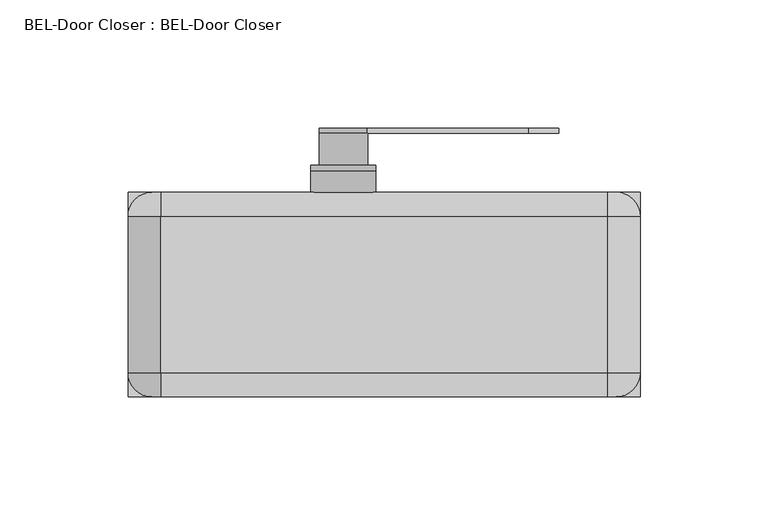
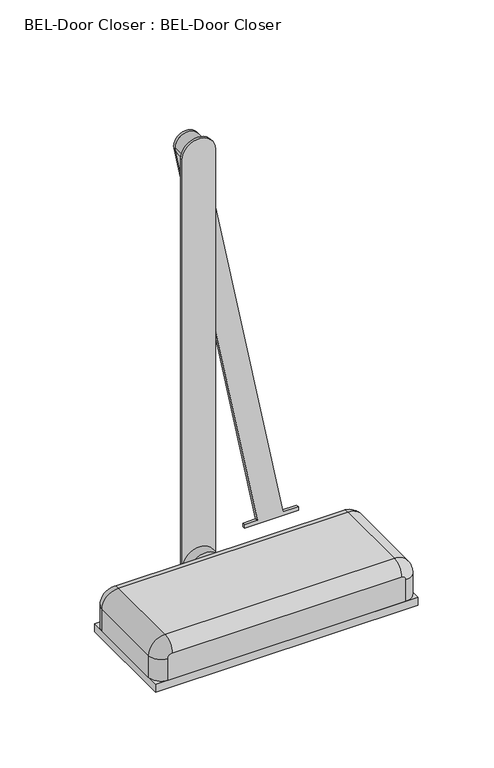
"""IFC4 building model written with IfcOpenShell, lengths in millimetres: proxy geometry, BEL-Door Closer : BEL-Door Closer."""

from ifc_helpers import new_model, si_unit, point, frame, frame_2d, origin, origin_with_axes, place, context, project, spatial, polyline, circle_curve, ellipse_curve, trimmed, segment, composite_curve, outline, extrude, source, transform, mapped, element, save
from ifc_brep_helpers import plane_surface, cylinder_surface, revolved_surface, advanced_brep


def bel_door_closer_bel_door_closer_a3520c2f(model_context):
    return source(origin(), model_context, "Body", "SolidModel", [
        extrude(outline(composite_curve([segment(trimmed(circle_curve(frame_2d((349.25, -273.05)), 9.525), [point((349.25, -282.575))], [point((349.25, -263.525))], False, "CARTESIAN"), True, "CONTINUOUS"), segment(trimmed(circle_curve(frame_2d((349.25, -273.05)), 9.525), [point((349.25, -263.525))], [point((349.25, -282.575))], False, "CARTESIAN"), True, "CONTINUOUS")], self_intersect=False)), frame((0.0, 32.6416667, 0.0), z_axis=(0.0, 1.0, 0.0), x_axis=(0.0, 0.0, 1.0)), (0.0, 0.0, 1.0), 12.5),
        extrude(outline(composite_curve([segment(trimmed(circle_curve(frame_2d((349.25, -273.0495842)), 9.5247276), [point((351.0696907, -263.7002975))], [point((347.4303363, -282.3988762))], False, "CARTESIAN"), True, "CONTINUOUS"), segment(polyline([(347.4303363, -282.3988762), (27.7698622, -220.1829834), (27.7542297, -229.9055371), (24.954228, -229.901035), (25.0199942, -188.9982584), (27.81999, -189.0027604), (27.8010501, -200.7822813), (351.0696907, -263.7002975)]), True, "CONTINUOUS")], self_intersect=False)), frame((0.0, 45.1416667, 0.0), z_axis=(0.0, 1.0, 0.0), x_axis=(0.0, 0.0, 1.0)), (0.0, 0.0, 1.0), 2.0833333),
        extrude(outline(composite_curve([segment(polyline([(5.475, -260.35), (349.25, -260.35)]), True, "CONTINUOUS"), segment(trimmed(circle_curve(frame_2d((349.25, -273.05)), 12.7), [point((349.25, -260.35))], [point((349.25, -285.75))], False, "CARTESIAN"), True, "CONTINUOUS"), segment(polyline([(349.25, -285.75), (5.475, -285.75), (5.475, -260.35)]), True, "CONTINUOUS")], self_intersect=False)), frame((0.0, 30.5583333, 0.0), z_axis=(0.0, 1.0, 0.0), x_axis=(0.0, 0.0, 1.0)), (0.0, 0.0, 1.0), 2.0833333),
        extrude(outline(composite_curve([segment(trimmed(circle_curve(frame_2d((21.35, -273.05)), 12.7), [point((21.35, -285.75))], [point((21.35, -260.35))], False, "CARTESIAN"), True, "CONTINUOUS"), segment(trimmed(circle_curve(frame_2d((21.35, -273.05)), 12.7), [point((21.35, -260.35))], [point((21.35, -285.75))], False, "CARTESIAN"), True, "CONTINUOUS")], self_intersect=False)), frame((0.0, 22.225, 0.0), z_axis=(0.0, 1.0, 0.0), x_axis=(0.0, 0.0, 1.0)), (0.0, 0.0, 1.0), 8.3333333),
        advanced_brep(
        [(-344.4875, 12.7000066, 36.35), (-344.4875, -48.25, 36.35), (-169.8875, -48.25, 36.35), (-169.8875, 12.7, 36.35), (-157.1875, 12.7, 6.35), (-157.1875, -48.25, 6.35), (-166.7125, -57.775, 6.35), (-347.6625, -57.775, 6.35), (-357.1875, -48.25, 6.35), (-357.1875, 12.7, 6.35), (-347.6625, 22.225, 6.35), (-166.7125, 22.225, 6.35), (-347.6625, 22.225, 23.65), (-344.4875, 22.225, 26.825), (-169.8875, 22.225, 26.825), (-166.7125, 22.225, 23.65), (-357.1875, -48.25, 23.65), (-357.1875, 12.7, 23.65), (-166.7125, -57.775, 23.65), (-169.8875, -57.775, 26.825), (-344.4875, -57.775, 26.825), (-347.6625, -57.775, 23.65), (-157.1875, 12.7, 23.65), (-157.1875, -48.25, 23.65)],
        [
            (0, 1),
            (1, 2),
            (2, 3),
            (3, 0),
            (4, 5),
            (5, 6, circle_curve(frame((-166.7125, -48.25, 6.35), z_axis=(0.0, 0.0, -1.0), x_axis=(-1.0, 0.0, 0.0)), 9.525)),
            (6, 7),
            (7, 8, circle_curve(frame((-347.6625, -48.25, 6.35), z_axis=(0.0, 0.0, -1.0), x_axis=(1.0, 0.0, 0.0)), 9.525)),
            (8, 9),
            (9, 10, circle_curve(frame((-347.6625, 12.7, 6.35), z_axis=(0.0, 0.0, -1.0), x_axis=(1.0, 0.0, 0.0)), 9.525)),
            (10, 11),
            (11, 4, circle_curve(frame((-166.7125, 12.7, 6.35), z_axis=(0.0, 0.0, -1.0), x_axis=(-1.0, 0.0, 0.0)), 9.525)),
            (10, 12),
            (12, 13, circle_curve(frame((-344.4875, 22.225, 23.65), z_axis=(0.0, 1.0, 0.0), x_axis=(-1.0, 0.0, 0.0)), 3.175)),
            (13, 14),
            (14, 15, circle_curve(frame((-169.8875, 22.225, 23.65), z_axis=(0.0, 1.0, 0.0), x_axis=(0.0, 0.0, 1.0)), 3.175)),
            (15, 11),
            (8, 16),
            (16, 17),
            (17, 9),
            (6, 18),
            (18, 19, circle_curve(frame((-169.8875, -57.775, 23.65), z_axis=(0.0, -1.0, 0.0), x_axis=(0.0, 0.0, 1.0)), 3.175)),
            (19, 20),
            (20, 21, circle_curve(frame((-344.4875, -57.775, 23.65), z_axis=(0.0, -1.0, 0.0), x_axis=(-1.0, 0.0, 0.0)), 3.175)),
            (21, 7),
            (4, 22),
            (22, 23),
            (23, 5),
            (0, 17, circle_curve(frame((-344.4875, 12.7, 23.65), z_axis=(0.0, -1.0, 0.0), x_axis=(1.0, 0.0, 0.0)), 12.7)),
            (16, 1, circle_curve(frame((-344.4875, -48.25, 23.65), z_axis=(0.0, 1.0, 0.0), x_axis=(1.0, 0.0, 0.0)), 12.7)),
            (2, 23, circle_curve(frame((-169.8875, -48.25, 23.65), z_axis=(0.0, 1.0, 0.0), x_axis=(1.0, 0.0, 0.0)), 12.7)),
            (22, 3, circle_curve(frame((-169.8875, 12.7, 23.65), z_axis=(0.0, -1.0, 0.0), x_axis=(1.0, 0.0, 0.0)), 12.7)),
            (17, 12, circle_curve(frame((-347.6625, 12.7, 23.65), z_axis=(0.0, 0.0, -1.0), x_axis=(1.0, 0.0, 0.0)), 9.525)),
            (21, 16, circle_curve(frame((-347.6625, -48.25, 23.65), z_axis=(0.0, 0.0, -1.0), x_axis=(1.0, 0.0, 0.0)), 9.525)),
            (0, 13, circle_curve(frame((-344.4875, 12.7, 26.825), z_axis=(-1.0, 0.0, 0.0), x_axis=(0.0, 0.0, -1.0)), 9.525)),
            (20, 1, circle_curve(frame((-344.4875, -48.25, 26.825), z_axis=(-1.0, 0.0, 0.0), x_axis=(0.0, 0.0, -1.0)), 9.525)),
            (3, 14, circle_curve(frame((-169.8875, 12.7, 26.825), z_axis=(-1.0, 0.0, 0.0), x_axis=(0.0, 0.0, -1.0)), 9.525)),
            (19, 2, circle_curve(frame((-169.8875, -48.25, 26.825), z_axis=(-1.0, 0.0, 0.0), x_axis=(0.0, 0.0, -1.0)), 9.525)),
            (22, 15, circle_curve(frame((-166.7125, 12.7, 23.65), z_axis=(0.0, 0.0, 1.0), x_axis=(-1.0, 0.0, 0.0)), 9.525)),
            (18, 23, circle_curve(frame((-166.7125, -48.25, 23.65), z_axis=(0.0, 0.0, 1.0), x_axis=(-1.0, 0.0, 0.0)), 9.525)),
        ],
        [
            plane_surface(frame((-357.1875, 22.225, 36.35), z_axis=(0.0, 0.0, 1.0), x_axis=(-1.0, 0.0, 0.0))),
            plane_surface(frame((-357.1875, 22.225, 6.35), z_axis=(0.0, 0.0, -1.0), x_axis=(1.0, 0.0, 0.0))),
            plane_surface(frame((-157.1875, 22.225, 36.35), z_axis=(0.0, 1.0, 0.0), x_axis=(0.0, 0.0, -1.0))),
            plane_surface(frame((-357.1875, 22.225, 36.35), z_axis=(-1.0, 0.0, 0.0), x_axis=(0.0, 0.0, -1.0))),
            plane_surface(frame((-357.1875, -57.775, 36.35), z_axis=(0.0, -1.0, 0.0), x_axis=(0.0, 0.0, -1.0))),
            plane_surface(frame((-157.1875, -57.775, 36.35), z_axis=(1.0, 0.0, 0.0), x_axis=(0.0, 0.0, -1.0))),
            cylinder_surface(frame((-344.4875, 22.225, 23.65), z_axis=(0.0, 1.0, 0.0), x_axis=(1.0, 0.0, 0.0)), 12.7),
            cylinder_surface(frame((-169.8875, -57.775, 23.65), z_axis=(0.0, 1.0, 0.0), x_axis=(1.0, 0.0, 0.0)), 12.7),
            cylinder_surface(frame((-347.6625, 12.7, 6.35), z_axis=(0.0, 0.0, 1.0), x_axis=(1.0, 0.0, 0.0)), 9.525),
            cylinder_surface(frame((-347.6625, -48.25, 6.35), z_axis=(0.0, 0.0, 1.0), x_axis=(1.0, 0.0, 0.0)), 9.525),
            revolved_surface(trimmed(ellipse_curve(frame((-347.6625, 12.7, 23.65), z_axis=(0.0, 0.0, -1.0), x_axis=(1.0, 0.0, 0.0)), 9.525, 9.525), [point((-357.1875, 12.7, 23.65))], [point((-347.6625, 22.225, 23.65))], True, "CARTESIAN"), (-344.4875, -57.775, 23.65), (0.0, 1.0, 0.0)),
            revolved_surface(trimmed(ellipse_curve(frame((-347.6625, -48.25, 23.65), z_axis=(0.0, 0.0, -1.0), x_axis=(1.0, 0.0, 0.0)), 9.525, 9.525), [point((-347.6625, -57.775, 23.65))], [point((-357.1875, -48.25, 23.65))], True, "CARTESIAN"), (-344.4875, -57.775, 23.65), (0.0, 1.0, 0.0)),
            cylinder_surface(frame((-344.4875, 12.7, 26.825), z_axis=(1.0, 0.0, 0.0), x_axis=(0.0, 0.0, -1.0)), 9.525),
            cylinder_surface(frame((-344.4875, -48.25, 26.825), z_axis=(1.0, 0.0, 0.0), x_axis=(0.0, 0.0, -1.0)), 9.525),
            revolved_surface(trimmed(ellipse_curve(frame((-169.8875, 12.7, 26.825), z_axis=(-1.0, 0.0, 0.0), x_axis=(0.0, 0.0, -1.0)), 9.525, 9.525), [point((-169.8875, 12.7, 36.35))], [point((-169.8875, 22.225, 26.825))], True, "CARTESIAN"), (-169.8875, -57.775, 23.65), (0.0, 1.0, 0.0)),
            revolved_surface(trimmed(ellipse_curve(frame((-169.8875, -48.25, 26.825), z_axis=(-1.0, 0.0, 0.0), x_axis=(0.0, 0.0, -1.0)), 9.525, 9.525), [point((-169.8875, -57.775, 26.825))], [point((-169.8875, -48.25, 36.35))], True, "CARTESIAN"), (-169.8875, -57.775, 23.65), (0.0, 1.0, 0.0)),
            cylinder_surface(frame((-166.7125, 12.7, 23.65), z_axis=(0.0, 0.0, -1.0), x_axis=(-1.0, 0.0, 0.0)), 9.525),
            cylinder_surface(frame((-166.7125, -48.25, 23.65), z_axis=(0.0, 0.0, -1.0), x_axis=(-1.0, 0.0, 0.0)), 9.525),
        ],
        [
            (0, [[1, 2, 3, 4]]),
            (1, [[5, 6, 7, 8, 9, 10, 11, 12]]),
            (2, [[-11, 13, 14, 15, 16, 17]]),
            (3, [[-9, 18, 19, 20]]),
            (4, [[-7, 21, 22, 23, 24, 25]]),
            (5, [[-5, 26, 27, 28]]),
            (6, [[-1, 29, -19, 30]]),
            (7, [[-3, 31, -27, 32]]),
            (8, [[33, -13, -10, -20]]),
            (9, [[34, -18, -8, -25]]),
            (10, [[-33, -29, 35, -14]]),
            (11, [[-34, -24, 36, -30]]),
            (12, [[-35, -4, 37, -15]]),
            (13, [[-36, -23, 38, -2]]),
            (14, [[-37, -32, 39, -16]]),
            (15, [[-38, -22, 40, -31]]),
            (16, [[-39, -26, -12, -17]]),
            (17, [[-40, -21, -6, -28]]),
        ],
    ),
        extrude(outline(polyline([(-157.1875, 22.225), (-157.1875, -57.775), (-357.1875, -57.775), (-357.1875, 22.225), (-157.1875, 22.225)])), origin_with_axes(), (0.0, 0.0, 1.0), 6.35),
    ])


if __name__ == "__main__":
    model = new_model("IFC4")
    model_context = context("Model", 3, world=origin())
    ifc_project = project(units=[si_unit("LENGTHUNIT", "METRE", prefix="MILLI")], contexts=[model_context])
    site = spatial("IfcSite", under=ifc_project)
    building = spatial("IfcBuilding", under=site)
    placement = place(None, origin())
    bel_door_closer_bel_door_closer_shape = bel_door_closer_bel_door_closer_a3520c2f(model_context)
    element("IfcBuildingElementProxy", 1, Name="BEL-Door Closer : BEL-Door Closer", ObjectType="BEL-Door Closer : BEL-Door Closer", at=placement, inside=building, context=model_context, shape_type="MappedRepresentation", body=[
        mapped(bel_door_closer_bel_door_closer_shape, transform((0.0, 0.0, 0.0), x_axis=(1.0, 0.0, 0.0), y_axis=(0.0, 1.0, 0.0), z_axis=(0.0, 0.0, 1.0))),
    ])
    save(model, "model.ifc")

# Revit data of these elements
# Type "BEL-Door Closer : BEL-Door Closer"
#   URL = "http://us.allegion.com/brands/falcon/Pages/default.aspx"
#   Standards Conformance = "as Specified"
#   Specification = ""
#   SpecWizard = ""
#   Send Message = "http://arcat.com/users.pl?action=UserEmail&company=Falcon+Lock&coid=32420&rep=114&fax=&mf="
#   Screw Pack Type = "as Specified"
#   Sales Information = "http://us.allegion.com/irst/Pages/contact_us.aspx"
#   Revision = "R1_02-2014"
#   Product Properties = ""
#   Product Data = "http://www.arcat.com/arcatcos/cos32/arc32420.html"
#   Model = "As Specified"
#   Manufacturer Website = "http://us.allegion.com/brands/falcon/Pages/default.aspx"
#   Manufacturer Phone = ""
#   Manufacturer Fax = ""
#   Manufacturer = "Falcon"
#   Keynote = "08710"
#   Installation-Fabrication = ""
#   Installation Phase = ""
#   Green Building-LEED = ""
#   Function Type = "as Specified"
#   Door Type = "as Specified"
#   Description = "Falcon Closer as Specified"
#   Copyright = "©Arcat Inc."
#   Construction Details = ""
#   Assembly Code = "C1020410"
#   originlocate [instance default] = 0' - 0"
#   locatearm [instance default] = 0' - 0 1/2"
#   Unit Width = 0' - 7.87402"
#   Unit Height = 0' - 3.14961"
#   Unit Depth = 0' - 1.1811"
#   Plate Thickness = 0' - 0 1/4"
#   Offset from Edge of Frame_Closer Arm [instance default] = 0' - 7"
#   Offset from Edge of Door_Closer Case [instance default] = 0' - 3 15/16"
#   Offset for Plate [instance default] = 0' - 0"
#   Reveal Between Door and Frame_Right [instance default] = 0' - 0 1/4"
#   Reveal Between Door and Frame_Left [instance default] = 0' - 0 1/4"
#   Door Leaf Width [instance default] = 3' - 0"
#   Door Leaf Top Reveal [instance default] = 0' - 0 1/4"
#   Door Leaf Thickness [instance default] = 0' - 0"
#   Closer Case Side Offset = 0' - 3 15/16"
#   Closer Arm Offset = 0' - 7"
#   Arm Width = 1' - 2"
#   Arm Height = 0' - 1 5/8"
#   Arm Extension [instance default] = 0' - 0"
#   Arm Depth = 1' - 2"
#   ActualArm Height [instance default] = 0' - 1 7/8"
#   ActualArm Depth [instance default] = 1' - 2"
#   Warranty Duration (Years) = 0
#   RH Hinge [instance default] = no
#   Maintenance Schedule (Months) = 0
#   LH Hinge [instance default] = yes
#   Include Mounting Plate [instance default] = no
#   Expected Lifespan (Years) = 0
#   Closer on Door Surface = yes
#   Closer on Door Frame = no
#   Arm Below Closer = no
#   Arm Above Closer = yes
#   Cover Material [instance default] = Metal - IR - Satin Chrome
#   Arm Type = element 418778
#   Arm Material [instance default] = Metal - IR - Satin Chrome
#   Default Elevation = 0
# Element 1 (IfcBuildingElementProxy, "BEL-Door Closer : BEL-Door Closer")
#   Offset for Plate = 0' - 0 1/4"
#   ActualArm Depth = 1' - 2 1/4"
#   Include Mounting Plate = yes
#   Materials on its faces: "Metal - IR - Satin Chrome"
# Materials
#   "Metal - IR - Satin Chrome": colour RGB 244 244 244, transparency 0, Cost = 0
